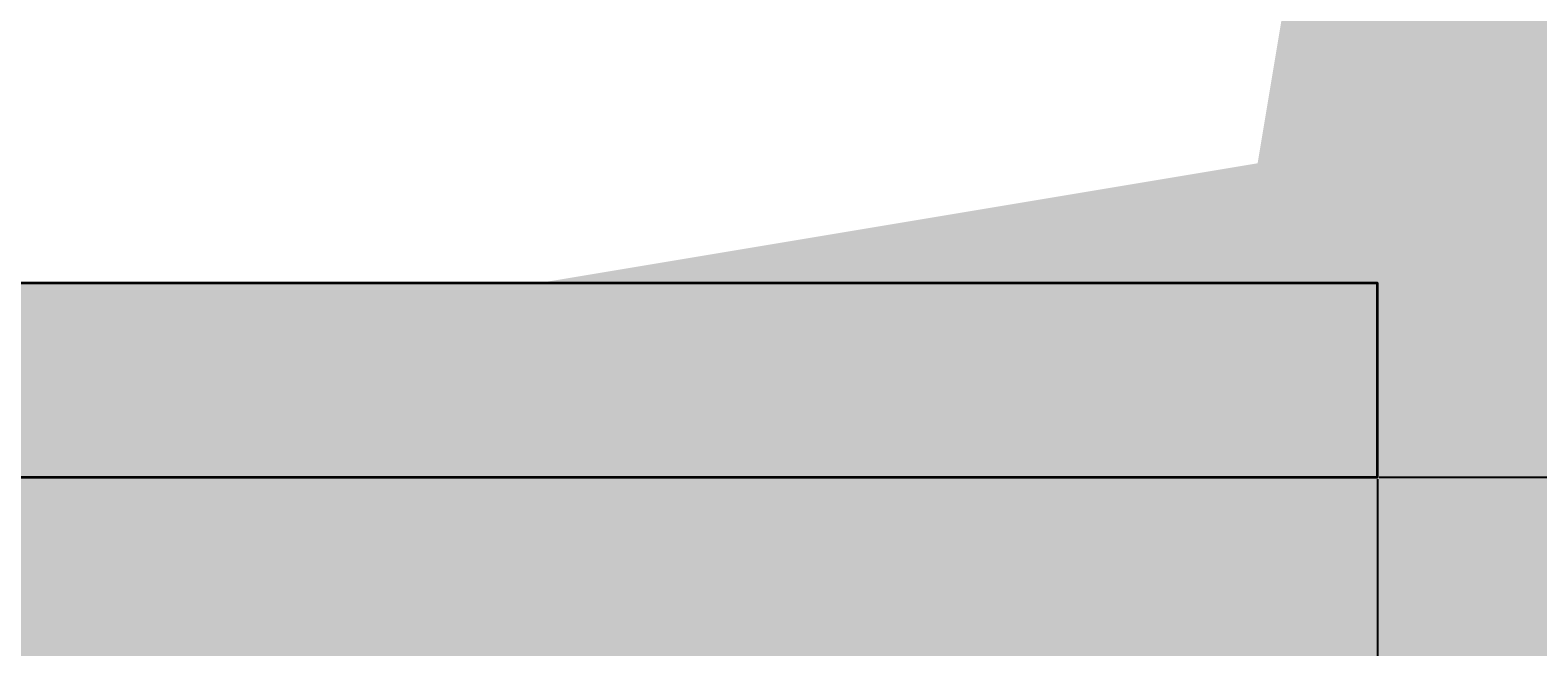
# Model space of a CAD drawing. Units: millimetres. Extents: x -22994 to 29398, y -19990 to 20176.
# Tile 55 of 135: x 247 to 296, y 5 to 25. Entities that reach past the tile are written whole.
import ezdxf

# ---------------------------------------------------------------- set-up
doc = ezdxf.new("R2010")
doc.units = ezdxf.units.MM
doc.header["$MEASUREMENT"] = 0
doc.layers.add('M-DIMS', color=2, linetype='Continuous', lineweight=18)
doc.layers.add('S-FNDN', color=7, linetype='Continuous', lineweight=35)
doc.styles.get("Standard").update_dxf_attribs({"font": 'arial.ttf'})
doc.dimstyles.get("Standard").update_dxf_attribs({"dimtxt": 0.18, "dimasz": 10000, "dimexe": 0.18, "dimexo": 0.0625, "dimgap": 0.09, "dimtad": 0, "dimtih": 1, "dimtoh": 1, "dimdec": 0, "dimzin": 0, "dimdsep": 46, "dimtxsty": 'Standard', "dimcen": 0.09, "dimadec": 0, "dimazin": 0, "dimtfac": 1, "dimtdec": 0, "dimtofl": 0, "dimtmove": 0, "dimatfit": 3, "dimfxl": 1, "dimtolj": 1, "dimtzin": 0, "dimlwd": 30, "dimarcsym": 0})

# ---------------------------------------------------------------- blocks, each defined once
blk = doc.blocks.new('*D2')
at = {"layer": 'Defpoints', "color": 0, "transparency": 16777216}
for p in [(6.677, 10.271), (290.852, 10.271), (290.852, -5.079)]:
    blk.add_point(p, dxfattribs=at)
at = {"layer": 'M-DIMS', "color": 0, "lineweight": -2, "transparency": 16777216}
for p, q in [((6.677, 10.209), (6.677, -5.259)), ((290.852, 10.209), (290.852, -5.259))]:
    blk.add_line(p, q, dxfattribs=at)
at = {"layer": 'M-DIMS', "color": 0, "lineweight": 30, "transparency": 16777216}
for p, q in [((-9993.323, -5.079), (-19993.323, -5.079)), ((10290.852, -5.079), (20290.852, -5.079))]:
    blk.add_line(p, q, dxfattribs=at)
at = {"layer": 'M-DIMS', "color": 0, "transparency": 16777216}
for points in [[(-9993.323, 1661.588), (-9993.323, -1671.745), (6.677, -5.079)], [(10290.852, 1661.588), (10290.852, -1671.745), (290.852, -5.079)]]:
    blk.add_solid(points, dxfattribs=at)
at = {"layer": 'M-DIMS', "color": 0, "transparency": 16777216, "insert": (148.765, -5.079), "char_height": 0.18, "attachment_point": 5}
blk.add_mtext('\\A1;284.2', dxfattribs=at)
blk = doc.blocks.new('*D3')
at = {"layer": 'Defpoints', "color": 0, "transparency": 16777216}
for p in [(110.265, 204.165), (110.265, 176.366), (95.833, 127.967)]:
    blk.add_point(p, dxfattribs=at)
at = {"layer": 'M-DIMS', "color": 0, "lineweight": -2, "transparency": 16777216}
for p, q in [((95.833, 128.03), (95.833, 204.345)), ((110.265, 176.429), (110.265, 204.345))]:
    blk.add_line(p, q, dxfattribs=at)
at = {"layer": 'M-DIMS', "color": 0, "lineweight": 30, "transparency": 16777216}
for p, q in [((-9904.167, 204.165), (-19904.167, 204.165)), ((10110.265, 204.165), (20110.265, 204.165))]:
    blk.add_line(p, q, dxfattribs=at)
at = {"layer": 'M-DIMS', "color": 0, "transparency": 16777216}
for points in [[(-9904.167, 1870.832), (-9904.167, -1462.501), (95.833, 204.165)], [(10110.265, 1870.832), (10110.265, -1462.501), (110.265, 204.165)]]:
    blk.add_solid(points, dxfattribs=at)
at = {"layer": 'M-DIMS', "color": 0, "transparency": 16777216, "insert": (103.049, 204.165), "char_height": 0.18, "attachment_point": 5}
blk.add_mtext('\\A1;14.432', dxfattribs=at)
blk = doc.blocks.new('*D4')
at = {"layer": 'Defpoints', "color": 0, "transparency": 16777216}
for p in [(116.265, 204.165), (110.265, 176.366), (116.265, 176.366)]:
    blk.add_point(p, dxfattribs=at)
at = {"layer": 'M-DIMS', "color": 0, "lineweight": -2, "transparency": 16777216}
for p, q in [((110.265, 176.429), (110.265, 204.345)), ((116.265, 176.429), (116.265, 204.345))]:
    blk.add_line(p, q, dxfattribs=at)
at = {"layer": 'M-DIMS', "color": 0, "lineweight": 30, "transparency": 16777216}
for p, q in [((-9889.735, 204.165), (-19889.735, 204.165)), ((10116.265, 204.165), (20116.265, 204.165))]:
    blk.add_line(p, q, dxfattribs=at)
at = {"layer": 'M-DIMS', "color": 0, "transparency": 16777216}
for points in [[(-9889.735, 1870.832), (-9889.735, -1462.501), (110.265, 204.165)], [(10116.265, 1870.832), (10116.265, -1462.501), (116.265, 204.165)]]:
    blk.add_solid(points, dxfattribs=at)
at = {"layer": 'M-DIMS', "color": 0, "transparency": 16777216, "insert": (113.265, 204.165), "char_height": 0.18, "attachment_point": 5}
blk.add_mtext('\\A1;6', dxfattribs=at)
blk = doc.blocks.new('*D5')
at = {"layer": 'Defpoints', "color": 0, "transparency": 16777216}
for p in [(181.265, 204.165), (116.265, 176.366), (181.265, 176.366)]:
    blk.add_point(p, dxfattribs=at)
at = {"layer": 'M-DIMS', "color": 0, "lineweight": -2, "transparency": 16777216}
for p, q in [((116.265, 176.429), (116.265, 204.345)), ((181.265, 176.429), (181.265, 204.345))]:
    blk.add_line(p, q, dxfattribs=at)
at = {"layer": 'M-DIMS', "color": 0, "lineweight": 30, "transparency": 16777216}
for p, q in [((-9883.735, 204.165), (-19883.735, 204.165)), ((10181.265, 204.165), (20181.265, 204.165))]:
    blk.add_line(p, q, dxfattribs=at)
at = {"layer": 'M-DIMS', "color": 0, "transparency": 16777216}
for points in [[(-9883.735, 1870.832), (-9883.735, -1462.501), (116.265, 204.165)], [(10181.265, 1870.832), (10181.265, -1462.501), (181.265, 204.165)]]:
    blk.add_solid(points, dxfattribs=at)
at = {"layer": 'M-DIMS', "color": 0, "transparency": 16777216, "insert": (148.765, 204.165), "char_height": 0.18, "attachment_point": 5}
blk.add_mtext('\\A1;65', dxfattribs=at)
blk = doc.blocks.new('*D6')
at = {"layer": 'Defpoints', "color": 0, "transparency": 16777216}
for p in [(187.265, 204.165), (181.265, 176.366), (187.265, 176.366)]:
    blk.add_point(p, dxfattribs=at)
at = {"layer": 'M-DIMS', "color": 0, "lineweight": -2, "transparency": 16777216}
for p, q in [((181.265, 176.429), (181.265, 204.345)), ((187.265, 176.429), (187.265, 204.345))]:
    blk.add_line(p, q, dxfattribs=at)
at = {"layer": 'M-DIMS', "color": 0, "lineweight": 30, "transparency": 16777216}
for p, q in [((-9818.735, 204.165), (-19818.735, 204.165)), ((10187.265, 204.165), (20187.265, 204.165))]:
    blk.add_line(p, q, dxfattribs=at)
at = {"layer": 'M-DIMS', "color": 0, "transparency": 16777216}
for points in [[(-9818.735, 1870.832), (-9818.735, -1462.501), (181.265, 204.165)], [(10187.265, 1870.832), (10187.265, -1462.501), (187.265, 204.165)]]:
    blk.add_solid(points, dxfattribs=at)
at = {"layer": 'M-DIMS', "color": 0, "transparency": 16777216, "insert": (184.265, 204.165), "char_height": 0.18, "attachment_point": 5}
blk.add_mtext('\\A1;6', dxfattribs=at)
blk = doc.blocks.new('*D7')
at = {"layer": 'Defpoints', "color": 0, "transparency": 16777216}
for p in [(201.697, 204.165), (187.265, 176.366), (201.697, 127.967)]:
    blk.add_point(p, dxfattribs=at)
at = {"layer": 'M-DIMS', "color": 0, "lineweight": -2, "transparency": 16777216}
for p, q in [((187.265, 176.429), (187.265, 204.345)), ((201.697, 128.03), (201.697, 204.345))]:
    blk.add_line(p, q, dxfattribs=at)
at = {"layer": 'M-DIMS', "color": 0, "lineweight": 30, "transparency": 16777216}
for p, q in [((-9812.735, 204.165), (-19812.735, 204.165)), ((10201.697, 204.165), (20201.697, 204.165))]:
    blk.add_line(p, q, dxfattribs=at)
at = {"layer": 'M-DIMS', "color": 0, "transparency": 16777216}
for points in [[(-9812.735, 1870.832), (-9812.735, -1462.501), (187.265, 204.165)], [(10201.697, 1870.832), (10201.697, -1462.501), (201.697, 204.165)]]:
    blk.add_solid(points, dxfattribs=at)
at = {"layer": 'M-DIMS', "color": 0, "transparency": 16777216, "insert": (194.481, 204.165), "char_height": 0.18, "attachment_point": 5}
blk.add_mtext('\\A1;14.432', dxfattribs=at)
blk = doc.blocks.new('*D8')
at = {"layer": 'Defpoints', "color": 0, "transparency": 16777216}
for p in [(227.648, 204.165), (227.648, 146.73), (201.697, 127.967)]:
    blk.add_point(p, dxfattribs=at)
at = {"layer": 'M-DIMS', "color": 0, "lineweight": -2, "transparency": 16777216}
for p, q in [((201.697, 128.03), (201.697, 204.345)), ((227.648, 146.792), (227.648, 204.345))]:
    blk.add_line(p, q, dxfattribs=at)
at = {"layer": 'M-DIMS', "color": 0, "lineweight": 30, "transparency": 16777216}
for p, q in [((-9798.303, 204.165), (-19798.303, 204.165)), ((10227.648, 204.165), (20227.648, 204.165))]:
    blk.add_line(p, q, dxfattribs=at)
at = {"layer": 'M-DIMS', "color": 0, "transparency": 16777216}
for points in [[(-9798.303, 1870.832), (-9798.303, -1462.501), (201.697, 204.165)], [(10227.648, 1870.832), (10227.648, -1462.501), (227.648, 204.165)]]:
    blk.add_solid(points, dxfattribs=at)
at = {"layer": 'M-DIMS', "color": 0, "transparency": 16777216, "insert": (214.673, 204.165), "char_height": 0.18, "attachment_point": 5}
blk.add_mtext('\\A1;25.95', dxfattribs=at)
blk = doc.blocks.new('*D9')
at = {"layer": 'Defpoints', "color": 0, "transparency": 16777216}
for p in [(187.265, 176.366), (306.202, 176.366), (290.852, 10.271)]:
    blk.add_point(p, dxfattribs=at)
at = {"layer": 'M-DIMS', "color": 0, "lineweight": 30, "transparency": 16777216}
for p, q in [((306.202, 10176.366), (306.202, 20176.366)), ((306.202, -9989.729), (306.202, -19989.729))]:
    blk.add_line(p, q, dxfattribs=at)
at = {"layer": 'M-DIMS', "color": 0, "lineweight": -2, "transparency": 16777216}
for p, q in [((187.327, 176.366), (306.382, 176.366)), ((290.915, 10.271), (306.382, 10.271))]:
    blk.add_line(p, q, dxfattribs=at)
at = {"layer": 'M-DIMS', "color": 0, "transparency": 16777216}
for points in [[(-1360.465, 10176.366), (1972.869, 10176.366), (306.202, 176.366)], [(-1360.465, -9989.729), (1972.869, -9989.729), (306.202, 10.271)]]:
    blk.add_solid(points, dxfattribs=at)
at = {"layer": 'M-DIMS', "color": 0, "transparency": 16777216, "insert": (306.202, 93.319), "char_height": 0.18, "attachment_point": 5}
blk.add_mtext('\\A1;166.1', dxfattribs=at)
blk = doc.blocks.new('*D10')
at = {"layer": 'Defpoints', "color": 0, "transparency": 16777216}
for p in [(125.65, 136.071), (133.346, 136.071), (133.346, -5.079)]:
    blk.add_point(p, dxfattribs=at)
at = {"layer": 'M-DIMS', "color": 0, "lineweight": -2, "transparency": 16777216}
for p, q in [((125.65, 136.009), (125.65, -5.259)), ((133.346, 136.009), (133.346, -5.259))]:
    blk.add_line(p, q, dxfattribs=at)
at = {"layer": 'M-DIMS', "color": 0, "lineweight": 30, "transparency": 16777216}
for p, q in [((-9874.35, -5.079), (-19874.35, -5.079)), ((10133.346, -5.079), (20133.346, -5.079))]:
    blk.add_line(p, q, dxfattribs=at)
at = {"layer": 'M-DIMS', "color": 0, "transparency": 16777216}
for points in [[(-9874.35, 1661.588), (-9874.35, -1671.745), (125.65, -5.079)], [(10133.346, 1661.588), (10133.346, -1671.745), (133.346, -5.079)]]:
    blk.add_solid(points, dxfattribs=at)
at = {"layer": 'M-DIMS', "color": 0, "transparency": 16777216, "insert": (129.498, -5.079), "char_height": 0.18, "attachment_point": 5}
blk.add_mtext('\\A1;7.696', dxfattribs=at)
blk = doc.blocks.new('*D11')
at = {"layer": 'Defpoints', "color": 0, "transparency": 16777216}
for p in [(133.346, 136.071), (135.65, 136.071), (135.65, -5.079)]:
    blk.add_point(p, dxfattribs=at)
at = {"layer": 'M-DIMS', "color": 0, "lineweight": -2, "transparency": 16777216}
for p, q in [((133.346, 136.009), (133.346, -5.259)), ((135.65, 136.009), (135.65, -5.259))]:
    blk.add_line(p, q, dxfattribs=at)
at = {"layer": 'M-DIMS', "color": 0, "lineweight": 30, "transparency": 16777216}
for p, q in [((-9866.654, -5.079), (-19866.654, -5.079)), ((10135.65, -5.079), (20135.65, -5.079))]:
    blk.add_line(p, q, dxfattribs=at)
at = {"layer": 'M-DIMS', "color": 0, "transparency": 16777216}
for points in [[(-9866.654, 1661.588), (-9866.654, -1671.745), (133.346, -5.079)], [(10135.65, 1661.588), (10135.65, -1671.745), (135.65, -5.079)]]:
    blk.add_solid(points, dxfattribs=at)
at = {"layer": 'M-DIMS', "color": 0, "transparency": 16777216, "insert": (134.498, -5.079), "char_height": 0.18, "attachment_point": 5}
blk.add_mtext('\\A1;2.304', dxfattribs=at)
blk = doc.blocks.new('*D12')
at = {"layer": 'Defpoints', "color": 0, "transparency": 16777216}
for p in [(135.65, 136.071), (145.65, 136.071), (145.65, -5.079)]:
    blk.add_point(p, dxfattribs=at)
at = {"layer": 'M-DIMS', "color": 0, "lineweight": -2, "transparency": 16777216}
for p, q in [((135.65, 136.009), (135.65, -5.259)), ((145.65, 136.009), (145.65, -5.259))]:
    blk.add_line(p, q, dxfattribs=at)
at = {"layer": 'M-DIMS', "color": 0, "lineweight": 30, "transparency": 16777216}
for p, q in [((-9864.35, -5.079), (-19864.35, -5.079)), ((10145.65, -5.079), (20145.65, -5.079))]:
    blk.add_line(p, q, dxfattribs=at)
at = {"layer": 'M-DIMS', "color": 0, "transparency": 16777216}
for points in [[(-9864.35, 1661.588), (-9864.35, -1671.745), (135.65, -5.079)], [(10145.65, 1661.588), (10145.65, -1671.745), (145.65, -5.079)]]:
    blk.add_solid(points, dxfattribs=at)
at = {"layer": 'M-DIMS', "color": 0, "transparency": 16777216, "insert": (140.65, -5.079), "char_height": 0.18, "attachment_point": 5}
blk.add_mtext('\\A1;10', dxfattribs=at)
blk = doc.blocks.new('*D13')
at = {"layer": 'Defpoints', "color": 0, "transparency": 16777216}
for p in [(145.65, 136.071), (155.65, 136.071), (155.65, -5.079)]:
    blk.add_point(p, dxfattribs=at)
at = {"layer": 'M-DIMS', "color": 0, "lineweight": -2, "transparency": 16777216}
for p, q in [((145.65, 136.009), (145.65, -5.259)), ((155.65, 136.009), (155.65, -5.259))]:
    blk.add_line(p, q, dxfattribs=at)
at = {"layer": 'M-DIMS', "color": 0, "lineweight": 30, "transparency": 16777216}
for p, q in [((-9854.35, -5.079), (-19854.35, -5.079)), ((10155.65, -5.079), (20155.65, -5.079))]:
    blk.add_line(p, q, dxfattribs=at)
at = {"layer": 'M-DIMS', "color": 0, "transparency": 16777216}
for points in [[(-9854.35, 1661.588), (-9854.35, -1671.745), (145.65, -5.079)], [(10155.65, 1661.588), (10155.65, -1671.745), (155.65, -5.079)]]:
    blk.add_solid(points, dxfattribs=at)
at = {"layer": 'M-DIMS', "color": 0, "transparency": 16777216, "insert": (150.65, -5.079), "char_height": 0.18, "attachment_point": 5}
blk.add_mtext('\\A1;10', dxfattribs=at)
blk = doc.blocks.new('*D14')
at = {"layer": 'Defpoints', "color": 0, "transparency": 16777216}
for p in [(155.65, 136.071), (165.65, 136.071), (165.65, -5.079)]:
    blk.add_point(p, dxfattribs=at)
at = {"layer": 'M-DIMS', "color": 0, "lineweight": -2, "transparency": 16777216}
for p, q in [((155.65, 136.009), (155.65, -5.259)), ((165.65, 136.009), (165.65, -5.259))]:
    blk.add_line(p, q, dxfattribs=at)
at = {"layer": 'M-DIMS', "color": 0, "lineweight": 30, "transparency": 16777216}
for p, q in [((-9844.35, -5.079), (-19844.35, -5.079)), ((10165.65, -5.079), (20165.65, -5.079))]:
    blk.add_line(p, q, dxfattribs=at)
at = {"layer": 'M-DIMS', "color": 0, "transparency": 16777216}
for points in [[(-9844.35, 1661.588), (-9844.35, -1671.745), (155.65, -5.079)], [(10165.65, 1661.588), (10165.65, -1671.745), (165.65, -5.079)]]:
    blk.add_solid(points, dxfattribs=at)
at = {"layer": 'M-DIMS', "color": 0, "transparency": 16777216, "insert": (160.65, -5.079), "char_height": 0.18, "attachment_point": 5}
blk.add_mtext('\\A1;10', dxfattribs=at)
blk = doc.blocks.new('*D15')
at = {"layer": 'Defpoints', "color": 0, "transparency": 16777216}
for p in [(173.346, 154.788), (173.346, 136.071), (306.202, 136.071)]:
    blk.add_point(p, dxfattribs=at)
at = {"layer": 'M-DIMS', "color": 0, "lineweight": 30, "transparency": 16777216}
for p, q in [((306.202, 10154.788), (306.202, 20154.788)), ((306.202, -9863.929), (306.202, -19863.929))]:
    blk.add_line(p, q, dxfattribs=at)
at = {"layer": 'M-DIMS', "color": 0, "lineweight": -2, "transparency": 16777216}
for p, q in [((173.408, 154.788), (306.382, 154.788)), ((173.408, 136.071), (306.382, 136.071))]:
    blk.add_line(p, q, dxfattribs=at)
at = {"layer": 'M-DIMS', "color": 0, "transparency": 16777216}
for points in [[(-1360.465, 10154.788), (1972.869, 10154.788), (306.202, 154.788)], [(-1360.465, -9863.929), (1972.869, -9863.929), (306.202, 136.071)]]:
    blk.add_solid(points, dxfattribs=at)
at = {"layer": 'M-DIMS', "color": 0, "transparency": 16777216, "insert": (306.202, 145.43), "char_height": 0.18, "attachment_point": 5}
blk.add_mtext('\\A1;18.717', dxfattribs=at)
blk = doc.blocks.new('*D16')
at = {"layer": 'Defpoints', "color": 0, "transparency": 16777216}
for p in [(120.17, 204.165), (110.466, 48.035), (120.17, 48.035)]:
    blk.add_point(p, dxfattribs=at)
at = {"layer": 'M-DIMS', "color": 0, "lineweight": -2, "transparency": 16777216}
for p, q in [((110.466, 48.097), (110.466, 204.345)), ((120.17, 48.097), (120.17, 204.345))]:
    blk.add_line(p, q, dxfattribs=at)
at = {"layer": 'M-DIMS', "color": 0, "lineweight": 30, "transparency": 16777216}
for p, q in [((-9889.534, 204.165), (-19889.534, 204.165)), ((10120.17, 204.165), (20120.17, 204.165))]:
    blk.add_line(p, q, dxfattribs=at)
at = {"layer": 'M-DIMS', "color": 0, "transparency": 16777216}
for points in [[(-9889.534, 1870.832), (-9889.534, -1462.501), (110.466, 204.165)], [(10120.17, 1870.832), (10120.17, -1462.501), (120.17, 204.165)]]:
    blk.add_solid(points, dxfattribs=at)
at = {"layer": 'M-DIMS', "color": 0, "transparency": 16777216, "insert": (115.318, 204.165), "char_height": 0.18, "attachment_point": 5}
blk.add_mtext('\\A1;9.704', dxfattribs=at)
blk = doc.blocks.new('*D17')
at = {"layer": 'Defpoints', "color": 0, "transparency": 16777216}
for p in [(126.17, 204.165), (120.17, 48.035), (126.17, 48.035)]:
    blk.add_point(p, dxfattribs=at)
at = {"layer": 'M-DIMS', "color": 0, "lineweight": -2, "transparency": 16777216}
for p, q in [((120.17, 48.097), (120.17, 204.345)), ((126.17, 48.097), (126.17, 204.345))]:
    blk.add_line(p, q, dxfattribs=at)
at = {"layer": 'M-DIMS', "color": 0, "lineweight": 30, "transparency": 16777216}
for p, q in [((-9879.83, 204.165), (-19879.83, 204.165)), ((10126.17, 204.165), (20126.17, 204.165))]:
    blk.add_line(p, q, dxfattribs=at)
at = {"layer": 'M-DIMS', "color": 0, "transparency": 16777216}
for points in [[(-9879.83, 1870.832), (-9879.83, -1462.501), (120.17, 204.165)], [(10126.17, 1870.832), (10126.17, -1462.501), (126.17, 204.165)]]:
    blk.add_solid(points, dxfattribs=at)
at = {"layer": 'M-DIMS', "color": 0, "transparency": 16777216, "insert": (123.17, 204.165), "char_height": 0.18, "attachment_point": 5}
blk.add_mtext('\\A1;6', dxfattribs=at)
blk = doc.blocks.new('*D18')
at = {"layer": 'Defpoints', "color": 0, "transparency": 16777216}
for p in [(132.17, 204.165), (126.17, 48.035), (132.17, 48.035)]:
    blk.add_point(p, dxfattribs=at)
at = {"layer": 'M-DIMS', "color": 0, "lineweight": -2, "transparency": 16777216}
for p, q in [((126.17, 48.097), (126.17, 204.345)), ((132.17, 48.097), (132.17, 204.345))]:
    blk.add_line(p, q, dxfattribs=at)
at = {"layer": 'M-DIMS', "color": 0, "lineweight": 30, "transparency": 16777216}
for p, q in [((-9873.83, 204.165), (-19873.83, 204.165)), ((10132.17, 204.165), (20132.17, 204.165))]:
    blk.add_line(p, q, dxfattribs=at)
at = {"layer": 'M-DIMS', "color": 0, "transparency": 16777216}
for points in [[(-9873.83, 1870.832), (-9873.83, -1462.501), (126.17, 204.165)], [(10132.17, 1870.832), (10132.17, -1462.501), (132.17, 204.165)]]:
    blk.add_solid(points, dxfattribs=at)
at = {"layer": 'M-DIMS', "color": 0, "transparency": 16777216, "insert": (129.17, 204.165), "char_height": 0.18, "attachment_point": 5}
blk.add_mtext('\\A1;6', dxfattribs=at)
blk = doc.blocks.new('*D19')
at = {"layer": 'Defpoints', "color": 0, "transparency": 16777216}
for p in [(138.17, 204.165), (132.17, 48.035), (138.17, 48.035)]:
    blk.add_point(p, dxfattribs=at)
at = {"layer": 'M-DIMS', "color": 0, "lineweight": -2, "transparency": 16777216}
for p, q in [((132.17, 48.097), (132.17, 204.345)), ((138.17, 48.097), (138.17, 204.345))]:
    blk.add_line(p, q, dxfattribs=at)
at = {"layer": 'M-DIMS', "color": 0, "lineweight": 30, "transparency": 16777216}
for p, q in [((-9867.83, 204.165), (-19867.83, 204.165)), ((10138.17, 204.165), (20138.17, 204.165))]:
    blk.add_line(p, q, dxfattribs=at)
at = {"layer": 'M-DIMS', "color": 0, "transparency": 16777216}
for points in [[(-9867.83, 1870.832), (-9867.83, -1462.501), (132.17, 204.165)], [(10138.17, 1870.832), (10138.17, -1462.501), (138.17, 204.165)]]:
    blk.add_solid(points, dxfattribs=at)
at = {"layer": 'M-DIMS', "color": 0, "transparency": 16777216, "insert": (135.17, 204.165), "char_height": 0.18, "attachment_point": 5}
blk.add_mtext('\\A1;6', dxfattribs=at)
blk = doc.blocks.new('*D20')
at = {"layer": 'Defpoints', "color": 0, "transparency": 16777216}
for p in [(144.17, 204.165), (138.17, 48.035), (144.17, 48.035)]:
    blk.add_point(p, dxfattribs=at)
at = {"layer": 'M-DIMS', "color": 0, "lineweight": -2, "transparency": 16777216}
for p, q in [((138.17, 48.097), (138.17, 204.345)), ((144.17, 48.097), (144.17, 204.345))]:
    blk.add_line(p, q, dxfattribs=at)
at = {"layer": 'M-DIMS', "color": 0, "lineweight": 30, "transparency": 16777216}
for p, q in [((-9861.83, 204.165), (-19861.83, 204.165)), ((10144.17, 204.165), (20144.17, 204.165))]:
    blk.add_line(p, q, dxfattribs=at)
at = {"layer": 'M-DIMS', "color": 0, "transparency": 16777216}
for points in [[(-9861.83, 1870.832), (-9861.83, -1462.501), (138.17, 204.165)], [(10144.17, 1870.832), (10144.17, -1462.501), (144.17, 204.165)]]:
    blk.add_solid(points, dxfattribs=at)
at = {"layer": 'M-DIMS', "color": 0, "transparency": 16777216, "insert": (141.17, 204.165), "char_height": 0.18, "attachment_point": 5}
blk.add_mtext('\\A1;6', dxfattribs=at)
blk = doc.blocks.new('*D21')
at = {"layer": 'Defpoints', "color": 0, "transparency": 16777216}
for p in [(149.116, 204.165), (144.17, 48.035), (149.116, 48.035)]:
    blk.add_point(p, dxfattribs=at)
at = {"layer": 'M-DIMS', "color": 0, "lineweight": -2, "transparency": 16777216}
for p, q in [((144.17, 48.097), (144.17, 204.345)), ((149.116, 48.097), (149.116, 204.345))]:
    blk.add_line(p, q, dxfattribs=at)
at = {"layer": 'M-DIMS', "color": 0, "lineweight": 30, "transparency": 16777216}
for p, q in [((-9855.83, 204.165), (-19855.83, 204.165)), ((10149.116, 204.165), (20149.116, 204.165))]:
    blk.add_line(p, q, dxfattribs=at)
at = {"layer": 'M-DIMS', "color": 0, "transparency": 16777216}
for points in [[(-9855.83, 1870.832), (-9855.83, -1462.501), (144.17, 204.165)], [(10149.116, 1870.832), (10149.116, -1462.501), (149.116, 204.165)]]:
    blk.add_solid(points, dxfattribs=at)
at = {"layer": 'M-DIMS', "color": 0, "transparency": 16777216, "insert": (146.643, 204.165), "char_height": 0.18, "attachment_point": 5}
blk.add_mtext('\\A1;4.945', dxfattribs=at)
blk = doc.blocks.new('*D22')
at = {"layer": 'Defpoints', "color": 0, "transparency": 16777216}
for p in [(149.116, 30.99), (155.116, 30.99), (155.116, -5.079)]:
    blk.add_point(p, dxfattribs=at)
at = {"layer": 'M-DIMS', "color": 0, "lineweight": -2, "transparency": 16777216}
for p, q in [((149.116, 30.927), (149.116, -5.259)), ((155.116, 30.927), (155.116, -5.259))]:
    blk.add_line(p, q, dxfattribs=at)
at = {"layer": 'M-DIMS', "color": 0, "lineweight": 30, "transparency": 16777216}
for p, q in [((-9850.884, -5.079), (-19850.884, -5.079)), ((10155.116, -5.079), (20155.116, -5.079))]:
    blk.add_line(p, q, dxfattribs=at)
at = {"layer": 'M-DIMS', "color": 0, "transparency": 16777216}
for points in [[(-9850.884, 1661.588), (-9850.884, -1671.745), (149.116, -5.079)], [(10155.116, 1661.588), (10155.116, -1671.745), (155.116, -5.079)]]:
    blk.add_solid(points, dxfattribs=at)
at = {"layer": 'M-DIMS', "color": 0, "transparency": 16777216, "insert": (152.116, -5.079), "char_height": 0.18, "attachment_point": 5}
blk.add_mtext('\\A1;6', dxfattribs=at)
blk = doc.blocks.new('*D23')
at = {"layer": 'Defpoints', "color": 0, "transparency": 16777216}
for p in [(155.116, 30.99), (161.116, 30.99), (161.116, -5.079)]:
    blk.add_point(p, dxfattribs=at)
at = {"layer": 'M-DIMS', "color": 0, "lineweight": -2, "transparency": 16777216}
for p, q in [((155.116, 30.927), (155.116, -5.259)), ((161.116, 30.927), (161.116, -5.259))]:
    blk.add_line(p, q, dxfattribs=at)
at = {"layer": 'M-DIMS', "color": 0, "lineweight": 30, "transparency": 16777216}
for p, q in [((-9844.884, -5.079), (-19844.884, -5.079)), ((10161.116, -5.079), (20161.116, -5.079))]:
    blk.add_line(p, q, dxfattribs=at)
at = {"layer": 'M-DIMS', "color": 0, "transparency": 16777216}
for points in [[(-9844.884, 1661.588), (-9844.884, -1671.745), (155.116, -5.079)], [(10161.116, 1661.588), (10161.116, -1671.745), (161.116, -5.079)]]:
    blk.add_solid(points, dxfattribs=at)
at = {"layer": 'M-DIMS', "color": 0, "transparency": 16777216, "insert": (158.116, -5.079), "char_height": 0.18, "attachment_point": 5}
blk.add_mtext('\\A1;6', dxfattribs=at)
blk = doc.blocks.new('*D24')
at = {"layer": 'Defpoints', "color": 0, "transparency": 16777216}
for p in [(161.116, 30.99), (166.439, 30.99), (166.439, -5.079)]:
    blk.add_point(p, dxfattribs=at)
at = {"layer": 'M-DIMS', "color": 0, "lineweight": -2, "transparency": 16777216}
for p, q in [((161.116, 30.927), (161.116, -5.259)), ((166.439, 30.927), (166.439, -5.259))]:
    blk.add_line(p, q, dxfattribs=at)
at = {"layer": 'M-DIMS', "color": 0, "lineweight": 30, "transparency": 16777216}
for p, q in [((-9838.884, -5.079), (-19838.884, -5.079)), ((10166.439, -5.079), (20166.439, -5.079))]:
    blk.add_line(p, q, dxfattribs=at)
at = {"layer": 'M-DIMS', "color": 0, "transparency": 16777216}
for points in [[(-9838.884, 1661.588), (-9838.884, -1671.745), (161.116, -5.079)], [(10166.439, 1661.588), (10166.439, -1671.745), (166.439, -5.079)]]:
    blk.add_solid(points, dxfattribs=at)
at = {"layer": 'M-DIMS', "color": 0, "transparency": 16777216, "insert": (163.777, -5.079), "char_height": 0.18, "attachment_point": 5}
blk.add_mtext('\\A1;5.323', dxfattribs=at)
blk = doc.blocks.new('*D25')
at = {"layer": 'Defpoints', "color": 0, "transparency": 16777216}
for p in [(166.439, 30.99), (172.439, 30.99), (172.439, -5.079)]:
    blk.add_point(p, dxfattribs=at)
at = {"layer": 'M-DIMS', "color": 0, "lineweight": -2, "transparency": 16777216}
for p, q in [((166.439, 30.927), (166.439, -5.259)), ((172.439, 30.927), (172.439, -5.259))]:
    blk.add_line(p, q, dxfattribs=at)
at = {"layer": 'M-DIMS', "color": 0, "lineweight": 30, "transparency": 16777216}
for p, q in [((-9833.561, -5.079), (-19833.561, -5.079)), ((10172.439, -5.079), (20172.439, -5.079))]:
    blk.add_line(p, q, dxfattribs=at)
at = {"layer": 'M-DIMS', "color": 0, "transparency": 16777216}
for points in [[(-9833.561, 1661.588), (-9833.561, -1671.745), (166.439, -5.079)], [(10172.439, 1661.588), (10172.439, -1671.745), (172.439, -5.079)]]:
    blk.add_solid(points, dxfattribs=at)
at = {"layer": 'M-DIMS', "color": 0, "transparency": 16777216, "insert": (169.439, -5.079), "char_height": 0.18, "attachment_point": 5}
blk.add_mtext('\\A1;6', dxfattribs=at)
blk = doc.blocks.new('*D26')
at = {"layer": 'Defpoints', "color": 0, "transparency": 16777216}
for p in [(172.439, 30.99), (178.439, 30.99), (178.439, -5.079)]:
    blk.add_point(p, dxfattribs=at)
at = {"layer": 'M-DIMS', "color": 0, "lineweight": -2, "transparency": 16777216}
for p, q in [((172.439, 30.927), (172.439, -5.259)), ((178.439, 30.927), (178.439, -5.259))]:
    blk.add_line(p, q, dxfattribs=at)
at = {"layer": 'M-DIMS', "color": 0, "lineweight": 30, "transparency": 16777216}
for p, q in [((-9827.561, -5.079), (-19827.561, -5.079)), ((10178.439, -5.079), (20178.439, -5.079))]:
    blk.add_line(p, q, dxfattribs=at)
at = {"layer": 'M-DIMS', "color": 0, "transparency": 16777216}
for points in [[(-9827.561, 1661.588), (-9827.561, -1671.745), (172.439, -5.079)], [(10178.439, 1661.588), (10178.439, -1671.745), (178.439, -5.079)]]:
    blk.add_solid(points, dxfattribs=at)
at = {"layer": 'M-DIMS', "color": 0, "transparency": 16777216, "insert": (175.439, -5.079), "char_height": 0.18, "attachment_point": 5}
blk.add_mtext('\\A1;6', dxfattribs=at)
blk = doc.blocks.new('*D27')
at = {"layer": 'Defpoints', "color": 0, "transparency": 16777216}
for p in [(178.439, 30.99), (188.117, 30.99), (188.117, -5.079)]:
    blk.add_point(p, dxfattribs=at)
at = {"layer": 'M-DIMS', "color": 0, "lineweight": -2, "transparency": 16777216}
for p, q in [((178.439, 30.927), (178.439, -5.259)), ((188.117, 30.927), (188.117, -5.259))]:
    blk.add_line(p, q, dxfattribs=at)
at = {"layer": 'M-DIMS', "color": 0, "lineweight": 30, "transparency": 16777216}
for p, q in [((-9821.561, -5.079), (-19821.561, -5.079)), ((10188.117, -5.079), (20188.117, -5.079))]:
    blk.add_line(p, q, dxfattribs=at)
at = {"layer": 'M-DIMS', "color": 0, "transparency": 16777216}
for points in [[(-9821.561, 1661.588), (-9821.561, -1671.745), (178.439, -5.079)], [(10188.117, 1661.588), (10188.117, -1671.745), (188.117, -5.079)]]:
    blk.add_solid(points, dxfattribs=at)
at = {"layer": 'M-DIMS', "color": 0, "transparency": 16777216, "insert": (183.278, -5.079), "char_height": 0.18, "attachment_point": 5}
blk.add_mtext('\\A1;9.679', dxfattribs=at)
blk = doc.blocks.new('*D28')
at = {"layer": 'Defpoints', "color": 0, "transparency": 16777216}
for p in [(188.117, 48.035), (306.202, 48.035), (188.117, 30.99)]:
    blk.add_point(p, dxfattribs=at)
at = {"layer": 'M-DIMS', "color": 0, "lineweight": 30, "transparency": 16777216}
for p, q in [((306.202, 10048.035), (306.202, 20048.035)), ((306.202, -9969.01), (306.202, -19969.01))]:
    blk.add_line(p, q, dxfattribs=at)
at = {"layer": 'M-DIMS', "color": 0, "lineweight": -2, "transparency": 16777216}
for p, q in [((188.18, 48.035), (306.382, 48.035)), ((188.18, 30.99), (306.382, 30.99))]:
    blk.add_line(p, q, dxfattribs=at)
at = {"layer": 'M-DIMS', "color": 0, "transparency": 16777216}
for points in [[(-1360.465, 10048.035), (1972.869, 10048.035), (306.202, 48.035)], [(-1360.465, -9969.01), (1972.869, -9969.01), (306.202, 30.99)]]:
    blk.add_solid(points, dxfattribs=at)
at = {"layer": 'M-DIMS', "color": 0, "transparency": 16777216, "insert": (306.202, 39.512), "char_height": 0.18, "attachment_point": 5}
blk.add_mtext('\\A1;17.045', dxfattribs=at)
blk = doc.blocks.new('*D29')
at = {"layer": 'Defpoints', "color": 0, "transparency": 16777216}
for p in [(36.801, 80.045), (64.03, 80.045)]:
    blk.add_point(p, dxfattribs=at)
at = {"layer": 'M-DIMS', "color": 0, "lineweight": -2, "transparency": 16777216}
for p, q in [((50.325, 80.045), (50.505, 80.045)), ((50.415, 79.955), (50.415, 80.135))]:
    blk.add_line(p, q, dxfattribs=at)
at = {"layer": 'M-DIMS', "color": 0, "lineweight": 30, "transparency": 16777216}
blk.add_line((20064.03, 80.03), (10064.03, 80.038), dxfattribs=at)
at = {"layer": 'M-DIMS', "color": 0, "transparency": 16777216}
blk.add_solid([(10064.031, 1746.704), (10064.028, -1586.629), (64.03, 80.045)], dxfattribs=at)
at = {"layer": 'M-DIMS', "color": 0, "transparency": 16777216, "insert": (20064.521, 80.03), "char_height": 0.18, "attachment_point": 5}
blk.add_mtext('\\A1;∅27.23', dxfattribs=at)
blk = doc.blocks.new('*D30')
at = {"layer": 'Defpoints', "color": 0, "transparency": 16777216}
for p in [(216.315, 146.729), (238.982, 146.73)]:
    blk.add_point(p, dxfattribs=at)
at = {"layer": 'M-DIMS', "color": 0, "lineweight": 30, "transparency": 16777216}
blk.add_line((20238.982, 147.496), (10238.982, 147.113), dxfattribs=at)
at = {"layer": 'M-DIMS', "color": 0, "lineweight": -2, "transparency": 16777216}
for p, q in [((227.558, 146.73), (227.738, 146.73)), ((227.648, 146.64), (227.648, 146.82))]:
    blk.add_line(p, q, dxfattribs=at)
at = {"layer": 'M-DIMS', "color": 0, "transparency": 16777216}
blk.add_solid([(10238.918, 1813.78), (10239.046, -1519.554), (238.982, 146.73)], dxfattribs=at)
at = {"layer": 'M-DIMS', "color": 0, "transparency": 16777216, "insert": (20239.544, 147.496), "char_height": 0.18, "attachment_point": 5}
blk.add_mtext('\\A1;∅22.667', dxfattribs=at)
blk = doc.blocks.new('*D31')
at = {"layer": 'Defpoints', "color": 0, "transparency": 16777216}
for p in [(223.164, 146.729), (232.133, 146.73)]:
    blk.add_point(p, dxfattribs=at)
at = {"layer": 'M-DIMS', "color": 0, "lineweight": 30, "transparency": 16777216}
blk.add_line((20232.133, 148.666), (10232.133, 147.698), dxfattribs=at)
at = {"layer": 'M-DIMS', "color": 0, "lineweight": -2, "transparency": 16777216}
for p, q in [((227.558, 146.73), (227.738, 146.73)), ((227.648, 146.64), (227.648, 146.82))]:
    blk.add_line(p, q, dxfattribs=at)
at = {"layer": 'M-DIMS', "color": 0, "transparency": 16777216}
blk.add_solid([(10231.971, 1814.364), (10232.294, -1518.969), (232.133, 146.73)], dxfattribs=at)
at = {"layer": 'M-DIMS', "color": 0, "transparency": 16777216, "insert": (20232.625, 148.666), "char_height": 0.18, "attachment_point": 5}
blk.add_mtext('\\A1;∅8.969', dxfattribs=at)
blk = doc.blocks.new('*D33')
at = {"layer": 'Defpoints', "color": 0, "transparency": 16777216}
for p in [(229.561, 154.377), (232.997, 153.351)]:
    blk.add_point(p, dxfattribs=at)
at = {"layer": 'M-DIMS', "color": 0, "lineweight": -2, "transparency": 16777216}
for p, q in [((229.471, 154.377), (229.651, 154.377)), ((229.561, 154.287), (229.561, 154.467))]:
    blk.add_line(p, q, dxfattribs=at)
at = {"layer": 'M-DIMS', "color": 0, "lineweight": 30, "transparency": 16777216}
for p, q in [((19396.339, -5570.838), (9814.668, -2708.743)), ((29396.339, -5570.838), (19396.339, -5570.838))]:
    blk.add_line(p, q, dxfattribs=at)
at = {"layer": 'M-DIMS', "color": 0, "transparency": 16777216}
blk.add_solid([(10291.684, -1111.798), (9337.652, -4305.689), (232.997, 153.351)], dxfattribs=at)
at = {"layer": 'M-DIMS', "color": 0, "transparency": 16777216, "insert": (29397.012, -5570.838), "char_height": 0.18, "attachment_point": 5}
blk.add_mtext('\\A1;6X R3.586', dxfattribs=at)
blk = doc.blocks.new('*D37')
at = {"layer": 'Defpoints', "color": 0, "transparency": 16777216}
for p in [(54.834, 118.615), (59.494, 118.614)]:
    blk.add_point(p, dxfattribs=at)
at = {"layer": 'M-DIMS', "color": 0, "lineweight": -2, "transparency": 16777216}
for p, q in [((57.074, 118.614), (57.254, 118.614)), ((57.164, 118.524), (57.164, 118.704))]:
    blk.add_line(p, q, dxfattribs=at)
at = {"layer": 'M-DIMS', "color": 0, "lineweight": 30, "transparency": 16777216}
blk.add_line((20059.493, 116.253), (10059.494, 117.434), dxfattribs=at)
at = {"layer": 'M-DIMS', "color": 0, "transparency": 16777216}
blk.add_solid([(10059.69, 1784.1), (10059.297, -1549.233), (59.494, 118.614)], dxfattribs=at)
at = {"layer": 'M-DIMS', "color": 0, "transparency": 16777216, "insert": (20059.985, 116.253), "char_height": 0.18, "attachment_point": 5}
blk.add_mtext('\\A1;∅4.659', dxfattribs=at)

msp = doc.modelspace()

# ---------------------------------------------------------------- hatches: boundary and pattern name
at = {"layer": 'S-FNDN'}
h = msp.add_hatch(color=256, dxfattribs=at)
h.set_gradient(color1=(241, 235, 31), color2=(244, 238, 81), tint=1, name='CYLINDER')
h.paths.add_polyline_path([(290.852, 16.6063), (201.6967, 16.6063), (95.8327, 16.6063), (81.8485, 16.6063), (82.3691, 10.2713), (290.852, 10.2713)])
h.paths.add_polyline_path([(81.8485, 16.6063), (60.8206, 16.6063), (62.0909, 10.2713), (82.3691, 10.2713)])
h.paths.add_polyline_path([(60.8206, 16.6063), (6.6773, 16.6063), (6.6773, 10.2713), (62.0909, 10.2713)])

# ---------------------------------------------------------------- linework, layer by layer
msp.add_lwpolyline([(95.8327, 16.6063), (6.6773, 16.6063), (6.6773, 10.2713), (290.852, 10.2713), (290.852, 16.6063), (201.6967, 16.6063)], dxfattribs=at)

# ---------------------------------------------------------------- dimensions: what is measured, and where the dimension line sits
at = {"layer": 'M-DIMS'}
for base, p1, p2, override, picture, middle in [((306.202, 176.3662), (290.852, 10.2713), (187.2647, 176.3662), {"dimdec": 1, "dimlfac": 1, "dimrnd": 0, "dimzin": 0, "dimdsep": 46, "dimlunit": 2}, '*D9', (306.202, 93.3187)), ((306.202, 136.0713), (173.3459, 154.788), (173.3459, 136.0713), {"dimdec": 3, "dimlfac": 1, "dimrnd": 0, "dimzin": 0, "dimdsep": 46, "dimlunit": 2}, '*D15', (306.202, 145.4297)), ((306.202, 48.0349), (188.1175, 30.9895), (188.1175, 48.0349), {"dimdec": 3, "dimlfac": 1, "dimrnd": 0, "dimzin": 0, "dimdsep": 46, "dimlunit": 2}, '*D28', (306.202, 39.5122))]:
    dim = msp.add_linear_dim(base=base, p1=p1, p2=p2, angle=90, dimstyle='Standard', override=override, dxfattribs=at)
    dim.commit()
    dim.dimension.update_dxf_attribs({"geometry": picture, "text_midpoint": middle})
for base, p1, p2, override, picture, middle in [((110.2647, 204.1654), (95.8327, 127.967), (110.2647, 176.3662), {"dimdec": 3, "dimlfac": 1, "dimrnd": 0, "dimzin": 0, "dimdsep": 46, "dimlunit": 2}, '*D3', (103.0487, 204.1654)), ((116.2647, 204.1654), (110.2647, 176.3662), (116.2647, 176.3662), {"dimdec": 0, "dimlfac": 1, "dimrnd": 0, "dimzin": 0, "dimdsep": 46, "dimlunit": 2}, '*D4', (113.2647, 204.1654)), ((120.1702, 204.1654), (110.4658, 48.0349), (120.1702, 48.0349), {"dimdec": 3, "dimlfac": 1, "dimrnd": 0, "dimzin": 0, "dimdsep": 46, "dimlunit": 2}, '*D16', (115.318, 204.1654)), ((181.2647, 204.1654), (116.2647, 176.3662), (181.2647, 176.3662), {"dimdec": 0, "dimlfac": 1, "dimrnd": 0, "dimzin": 0, "dimdsep": 46, "dimlunit": 2}, '*D5', (148.7647, 204.1654)), ((126.1702, 204.1654), (120.1702, 48.0349), (126.1702, 48.0349), {"dimdec": 0, "dimlfac": 1, "dimrnd": 0, "dimzin": 0, "dimdsep": 46, "dimlunit": 2}, '*D17', (123.1702, 204.1654)), ((132.1702, 204.1654), (126.1702, 48.0349), (132.1702, 48.0349), {"dimdec": 0, "dimlfac": 1, "dimrnd": 0, "dimzin": 0, "dimdsep": 46, "dimlunit": 2}, '*D18', (129.1702, 204.1654)), ((138.1702, 204.1654), (132.1702, 48.0349), (138.1702, 48.0349), {"dimdec": 0, "dimlfac": 1, "dimrnd": 0, "dimzin": 0, "dimdsep": 46, "dimlunit": 2}, '*D19', (135.1702, 204.1654)), ((144.1702, 204.1654), (138.1702, 48.0349), (144.1702, 48.0349), {"dimdec": 0, "dimlfac": 1, "dimrnd": 0, "dimzin": 0, "dimdsep": 46, "dimlunit": 2}, '*D20', (141.1702, 204.1654)), ((149.11567, 204.16539), (144.17023, 48.03494), (149.11567, 48.03494), {"dimdec": 3, "dimlfac": 1, "dimrnd": 0, "dimzin": 0, "dimdsep": 46, "dimlunit": 2}, '*D21', (146.64295, 204.16539)), ((187.2647, 204.1654), (181.2647, 176.3662), (187.2647, 176.3662), {"dimdec": 0, "dimlfac": 1, "dimrnd": 0, "dimzin": 0, "dimdsep": 46, "dimlunit": 2}, '*D6', (184.2647, 204.1654)), ((201.6967, 204.1654), (187.2647, 176.3662), (201.6967, 127.967), {"dimdec": 3, "dimlfac": 1, "dimrnd": 0, "dimzin": 0, "dimdsep": 46, "dimlunit": 2}, '*D7', (194.4807, 204.1654)), ((227.6485, 204.1654), (201.6967, 127.967), (227.6485, 146.7296), {"dimdec": 2, "dimlfac": 1, "dimrnd": 0, "dimzin": 0, "dimdsep": 46, "dimlunit": 2}, '*D8', (214.6726, 204.1654)), ((290.852, -5.0787), (6.6773, 10.2713), (290.852, 10.2713), {"dimdec": 1, "dimlfac": 1, "dimrnd": 0, "dimzin": 0, "dimdsep": 46, "dimlunit": 2}, '*D2', (148.7647, -5.0787)), ((133.3459, -5.0787), (125.6498, 136.0713), (133.3459, 136.0713), {"dimdec": 3, "dimlfac": 1, "dimrnd": 0, "dimzin": 0, "dimdsep": 46, "dimlunit": 2}, '*D10', (129.4978, -5.0787)), ((135.6498, -5.0787), (133.3459, 136.0713), (135.6498, 136.0713), {"dimdec": 3, "dimlfac": 1, "dimrnd": 0, "dimzin": 0, "dimdsep": 46, "dimlunit": 2}, '*D11', (134.4978, -5.0787)), ((145.6498, -5.0787), (135.6498, 136.0713), (145.6498, 136.0713), {"dimdec": 0, "dimlfac": 1, "dimrnd": 0, "dimzin": 0, "dimdsep": 46, "dimlunit": 2}, '*D12', (140.6498, -5.0787)), ((155.6498, -5.0787), (145.6498, 136.0713), (155.6498, 136.0713), {"dimdec": 0, "dimlfac": 1, "dimrnd": 0, "dimzin": 0, "dimdsep": 46, "dimlunit": 2}, '*D13', (150.6498, -5.0787)), ((155.1157, -5.0787), (149.1157, 30.9895), (155.1157, 30.9895), {"dimdec": 0, "dimlfac": 1, "dimrnd": 0, "dimzin": 0, "dimdsep": 46, "dimlunit": 2}, '*D22', (152.1157, -5.0787)), ((161.1157, -5.0787), (155.1157, 30.9895), (161.1157, 30.9895), {"dimdec": 0, "dimlfac": 1, "dimrnd": 0, "dimzin": 0, "dimdsep": 46, "dimlunit": 2}, '*D23', (158.1157, -5.0787)), ((165.6498, -5.0787), (155.6498, 136.0713), (165.6498, 136.0713), {"dimdec": 0, "dimlfac": 1, "dimrnd": 0, "dimzin": 0, "dimdsep": 46, "dimlunit": 2}, '*D14', (160.6498, -5.0787)), ((166.4387, -5.0787), (161.1157, 30.9895), (166.4387, 30.9895), {"dimdec": 3, "dimlfac": 1, "dimrnd": 0, "dimzin": 0, "dimdsep": 46, "dimlunit": 2}, '*D24', (163.7772, -5.0787)), ((172.4387, -5.0787), (166.4387, 30.9895), (172.4387, 30.9895), {"dimdec": 0, "dimlfac": 1, "dimrnd": 0, "dimzin": 0, "dimdsep": 46, "dimlunit": 2}, '*D25', (169.4387, -5.0787)), ((178.4387, -5.0787), (172.4387, 30.9895), (178.4387, 30.9895), {"dimdec": 0, "dimlfac": 1, "dimrnd": 0, "dimzin": 0, "dimdsep": 46, "dimlunit": 2}, '*D26', (175.4387, -5.0787)), ((188.1175, -5.0787), (178.4387, 30.9895), (188.1175, 30.9895), {"dimdec": 3, "dimlfac": 1, "dimrnd": 0, "dimzin": 0, "dimdsep": 46, "dimlunit": 2}, '*D27', (183.2781, -5.0787))]:
    dim = msp.add_linear_dim(base=base, p1=p1, p2=p2, dimstyle='Standard', override=override, dxfattribs=at)
    dim.commit()
    dim.dimension.update_dxf_attribs({"geometry": picture, "text_midpoint": middle})
for p1, p2, picture, middle in [((223.1641, 146.7291), (232.1328, 146.73), '*D31', (20232.1327, 148.6656)), ((216.3148, 146.7291), (238.9821, 146.73), '*D30', (20238.9821, 147.4959))]:
    dim = msp.add_diameter_dim_2p(p1=p1, p2=p2, dimstyle='Standard', override={"dimdec": 3, "dimlfac": 1, "dimrnd": 0, "dimzin": 0, "dimdsep": 46, "dimlunit": 2}, dxfattribs=at)
    dim.commit()
    dim.dimension.update_dxf_attribs({"geometry": picture, "text_midpoint": middle, "dimtype": 163})
for p1, p2, override, picture, middle in [((54.8343, 118.6145), (59.4936, 118.614), {"dimdec": 3, "dimlfac": 1, "dimrnd": 0, "dimzin": 0, "dimdsep": 46, "dimlunit": 2}, '*D37', (20059.4934, 116.2531)), ((36.8006, 80.045), (64.0296, 80.045), {"dimdec": 2, "dimlfac": 1, "dimrnd": 0, "dimzin": 0, "dimdsep": 46, "dimlunit": 2}, '*D29', (20064.0296, 80.0303))]:
    dim = msp.add_diameter_dim_2p(p1=p1, p2=p2, dimstyle='Standard', override=override, dxfattribs=at)
    dim.commit()
    dim.dimension.update_dxf_attribs({"geometry": picture, "text_midpoint": middle})
dim = msp.add_radius_dim(center=(229.5613, 154.3773), mpoint=(232.9972, 153.3509), text='6X <>', dimstyle='Standard', override={"dimdec": 3, "dimlfac": 1, "dimrnd": 0, "dimzin": 0, "dimdsep": 46, "dimlunit": 2}, dxfattribs=at)
dim.commit()
dim.dimension.update_dxf_attribs({"geometry": '*D33', "text_midpoint": (29397.0125, -5570.8378)})

doc.saveas('drawing.dxf')
